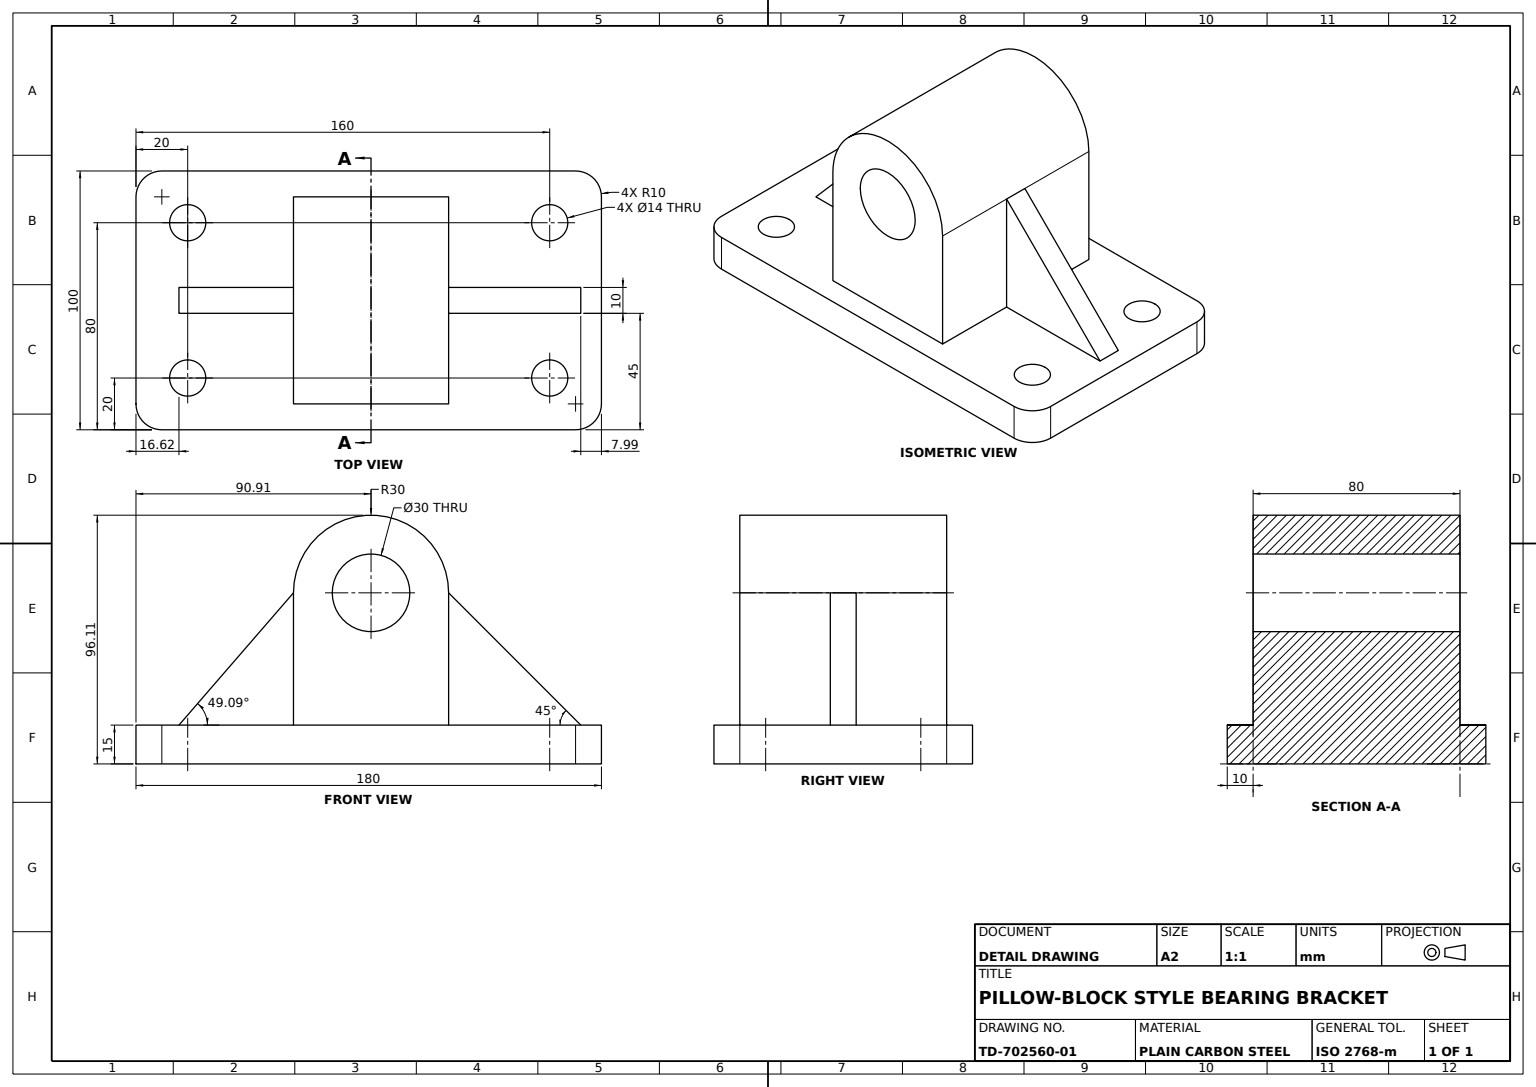
SolidWorks part; units mm, degrees
material "Plain Carbon Steel"
ref_plane "Front Plane" through (0, 0, 0) normal (0, 0, 1) x (1, 0, 0)
ref_plane "Top Plane" through (0, 0, 0) normal (0, 1, 0) x (1, 0, 0)
ref_plane "Right Plane" through (0, 0, 0) normal (1, 0, 0) x (0, 0, -1)
sketch "Base Plate Sketch" plane through (0, 0, 0) normal (0, 0, 1) x (1, 0, 0)
  line L0 (0, 0) -> (180, 0)
  line L1 (180, 0) -> (180, 15)
  line L2 (180, 15) -> (0, 15)
  line L3 (0, 15) -> (0, 0)
  dimension "D1" = 180
  dimension "D2" = 15
extrude "Base Plate" add sketch "Base Plate Sketch" along normal blind 100
ref_plane "Plane1" through (0, 0, 50) normal (0, 0, 1) x (1, 0, 0)
sketch "Bearing Upright Sketch" plane through (0, 0, 50) normal (0, 0, 1) x (1, 0, 0)
  line L0 (90.9059, 16.1059) -> (90.9059, 66.1059) construction
  line L1 (60.9059, 66.1059) -> (60.9059, 16.1059)
  line L2 (120.9059, 66.1059) -> (120.9059, 16.1059)
  line L3 (60.9059, 16.1059) -> (120.9059, 16.1059)
  circle A0 centre (90.9059, 66.1059) radius 15
  circle A1 centre (90.9059, 66.1059) radius 30
  dimension "D1" = 30
  dimension "D2" = 60
  dimension "D3" = 50
  dimension "D4" = 90.9059
  dimension "D5" = 16.1059
extrude "Bearing Upright" add sketch "Bearing Upright Sketch" against normal mid plane 80 separate body contours A0 | A1
sketch "Upright Block Sketch" plane through (0, 0, 50) normal (0, 0, 1) x (1, 0, 0)
  line L0 (60.9059, 66.1059) -> (60.9059, 15)
  line L1 (180, 15) -> (0, 15) construction
  line L2 (60.9059, 15) -> (120.9059, 15)
  line L3 (120.9059, 15) -> (120.9059, 66.1059)
  line L4 (60.9059, 66.1059) -> (120.9059, 66.1059)
  circle A0 centre (90.9059, 66.1059) radius 30 construction
  dimension "D1" = 60
extrude "Upright Block" add sketch "Upright Block Sketch" along normal mid plane 80
sketch "Bearing Bore Sketch" plane through (0, 0, 90) normal (0, 0, 1) x (1, 0, 0)
  line L0 (105.9059, 66.1059) -> (75.9059, 66.1059) construction
  circle A0 centre (90.9059, 66.1059) radius 15
  dimension "D1" = 30
extrude "Bearing Bore" cut sketch "Bearing Bore Sketch" against normal blind 80
ref_plane "Plane2" through (0, 0, 50) normal (0, 0, 1) x (1, 0, 0)
ref_plane "Plane4" through (0, 0, 50) normal (0, 0, 1) x (1, 0, 0)
sketch "Support Rib A Sketch" plane through (0, 0, 50) normal (0, 0, 1) x (1, 0, 0)
  line L0 (60.9059, 66.1059) -> (15.0663, 13.2028)
  dimension "D1" = 45.8395
  dimension "D2" = 52.9031
rib "Support Rib A" sketch "Support Rib A Sketch" sketch "Support Rib A Sketch" thickness 10 extrusion direction parallel to sketch draft on no parameters "D1"=10
sketch "Support Rib B Sketch" plane through (0, 0, 50) normal (0, 0, 1) x (1, 0, 0)
  line L0 (120.9059, 66.1059) -> (170.4034, 16.6084)
  dimension "D1" = 49.4975
  dimension "D2" = 49.4975
rib "Support Rib B" sketch "Support Rib B Sketch" sketch "Support Rib B Sketch" thickness 10 extrusion direction parallel to sketch draft on no parameters "D1"=10
sketch "Base Plate Cut A Sketch" plane through (0, 15, 0) normal (0, 1, 0) x (1, 0, 0)
  line L0 (0, 0) -> (20, 0) construction
  line L1 (180, 0) -> (0, 0) construction
  line L2 (20, 0) -> (20, -20) construction
  line L3 (0, -100) -> (0, 0) construction
  circle A0 centre (20, -20) radius 7
  dimension "D1" = 14
  dimension "D2" = 20
extrude "Base Plate Cut A" cut sketch "Base Plate Cut A Sketch" against normal blind 80
sketch "Base Plate Cut B Sketch" plane through (0, 15, 0) normal (0, 1, 0) x (1, 0, 0)
  line L0 (0, -100) -> (0, 0) construction
  line L1 (180, -100) -> (0, -100) construction
  circle A0 centre (160, -20) radius 7
  circle A1 centre (160, -80) radius 7
  circle A2 centre (20, -80) radius 7
  dimension "D1" = 14
  dimension "D2" = 20
  dimension "D3" = 160
  dimension "D4" = 20
  dimension "D5" = 80
extrude "Base Plate Cut B" cut sketch "Base Plate Cut B Sketch" against normal through all
fillet "Base Plate Corner Fillets R10" radius 10 4 edges at (0, 7.5, 0) (180, 7.5, 0) (180, 7.5, 100) (0, 7.5, 100)
